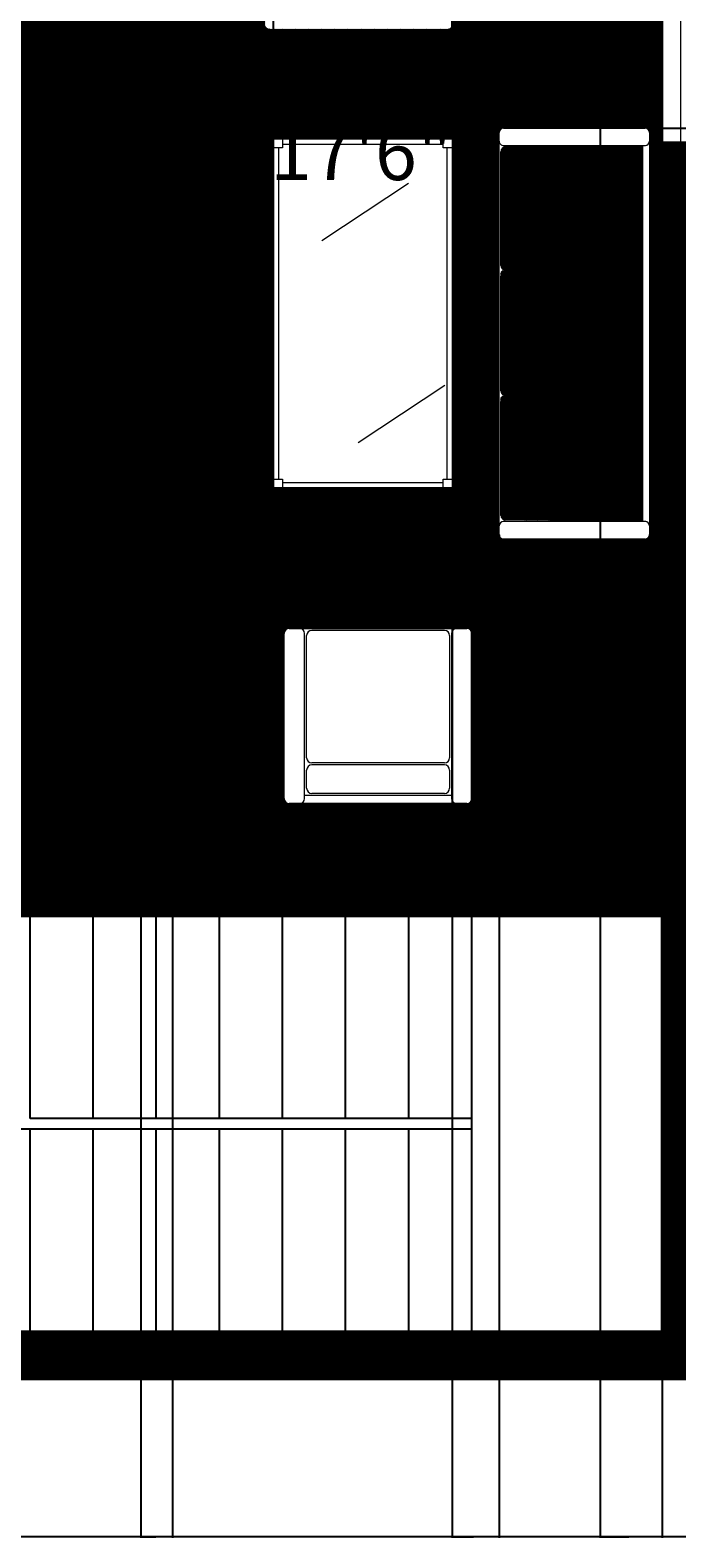
# Model space of a CAD drawing. Units: inches. Extents: x 205 to 1667, y -23 to 828.
# Tile 4 of 10: x 645 to 768, y -23 to 264. Entities that reach past the tile are written whole.
import ezdxf

# ---------------------------------------------------------------- set-up
doc = ezdxf.new("R2010")
doc.units = ezdxf.units.IN
doc.header["$MEASUREMENT"] = 0
for name, color, linetype, lineweight in [('A-ANNO-DIMS', 2, 'Continuous', 18), ('A-AREA-IDEN', 7, 'Continuous', 25), ('A-FLOR-STRS', 7, 'Continuous', 25), ('A-FURN', 8, 'Continuous', 18), ('A-GLAZ', 4, 'Continuous', 18), ('A-WALL', 7, 'Continuous', 35)]:
    doc.layers.add(name, color=color, linetype=linetype, lineweight=lineweight)
doc.layers.add('A-FLOR-PATT', color=9, linetype='Continuous', lineweight=9, true_color=0xc7c8ca)
doc.styles.get("Standard").update_dxf_attribs({"font": 'arial.ttf'})
doc.dimstyles.get("Standard").update_dxf_attribs({"dimtxt": 0.18, "dimasz": 0.18, "dimexe": 0.18, "dimexo": 0.0625, "dimgap": 0.09, "dimtad": 0, "dimtih": 1, "dimtoh": 1, "dimdec": 4, "dimzin": 0, "dimdsep": 46, "dimtxsty": 'Standard', "dimcen": 0.09, "dimadec": 0, "dimazin": 0, "dimtfac": 1, "dimtdec": 4, "dimtofl": 0, "dimtmove": 0, "dimatfit": 3, "dimfxl": 1, "dimtolj": 1, "dimtzin": 0, "dimarcsym": 0})

# ---------------------------------------------------------------- blocks, each defined once
blk = doc.blocks.new('A$C0BA509B0')
for p, q in [((0, 0.025), (0, 0.835)), ((0.025, 0.86), (2.325, 0.86)), ((0.1, 0.0219), (0.1, 0.8375)), ((0.1, 0.82), (2.25, 0.82)), ((0.11, 0.695), (0.11, 0.785)), ((0.135, 0.81), (0.7866, 0.81)), ((0.8116, 0.785), (0.8116, 0.695)), ((0.8216, 0.785), (0.8216, 0.695)), ((0.8466, 0.81), (1.5033, 0.81)), ((1.5283, 0.785), (1.5283, 0.695)), ((1.5383, 0.785), (1.5383, 0.695)), ((1.5633, 0.81), (2.215, 0.81)), ((2.24, 0.785), (2.24, 0.695)), ((2.25, 0.8385), (2.25, 0.0224)), ((2.35, 0.835), (2.35, 0.025)), ((0.11, 0.035), (0.11, 0.635)), ((0.135, 0.67), (0.7866, 0.67)), ((0.135, 0.66), (0.7866, 0.66)), ((0.8116, 0.635), (0.8116, 0.035)), ((0.8216, 0.635), (0.8216, 0.035)), ((0.8466, 0.67), (1.5033, 0.67)), ((0.8466, 0.66), (1.5033, 0.66)), ((1.5283, 0.635), (1.5283, 0.035)), ((1.5383, 0.635), (1.5383, 0.035)), ((1.5633, 0.67), (2.215, 0.67)), ((1.5633, 0.66), (2.215, 0.66)), ((2.24, 0.635), (2.24, 0.035)), ((0.7866, 0.01), (0.135, 0.01)), ((1.5033, 0.01), (0.8466, 0.01)), ((2.215, 0.01), (1.5633, 0.01)), ((2.325, 0), (0.025, 0))]:
    blk.add_line(p, q)
for centre, start, end in [((0.025, 0.835), 90, 180), ((0.0751, 0.835), 0, 90), ((0.135, 0.785), 90, 180), ((0.7866, 0.785), 0, 90), ((0.8466, 0.785), 90, 180), ((1.5033, 0.785), 0, 90), ((1.5633, 0.785), 90, 180), ((2.215, 0.785), 0, 90), ((2.2752, 0.835), 90, 180), ((2.325, 0.835), 0, 90), ((0.135, 0.695), 180, 270), ((0.7866, 0.695), 270, 0), ((0.8466, 0.695), 180, 270), ((1.5033, 0.695), 270, 0), ((1.5633, 0.695), 180, 270), ((2.215, 0.695), 270, 0), ((0.135, 0.635), 90, 180), ((0.7866, 0.635), 0, 90), ((0.8466, 0.635), 90, 180), ((1.5033, 0.635), 0, 90), ((1.5633, 0.635), 90, 180), ((2.215, 0.635), 0, 90), ((0.025, 0.025), 180, 270), ((0.0751, 0.025), 270, 0), ((0.135, 0.035), 180, 270), ((0.7866, 0.035), 270, 0), ((0.8466, 0.035), 180, 270), ((1.5033, 0.035), 270, 0), ((1.5633, 0.035), 180, 270), ((2.215, 0.035), 270, 0), ((2.2749, 0.025), 180, 270), ((2.325, 0.025), 270, 0)]:
    blk.add_arc(centre, 0.025, start, end)
blk = doc.blocks.new('WIN-48IN')
for p, q in [((0, 0), (0, 9)), ((0, 9), (48, 9)), ((48, 9), (48, 0)), ((48, 5.5), (0, 5.5)), ((48, 3.5), (0, 3.5)), ((48, 0), (0, 0))]:
    blk.add_line(p, q)
blk = doc.blocks.new('CHAIR-LOUNGE')
for p, q in [((0, 0.97), (0, 32.36)), ((0.97, 33.33), (34.75, 33.33)), ((3.88, 0.83), (3.88, 32.46)), ((4.26, 8.72), (4.26, 31.94)), ((30.48, 32.94), (5.26, 32.94)), ((31.45, 31.97), (31.45, 8.72)), ((31.84, 32.48), (31.84, 0.87)), ((35.71, 32.36), (35.71, 0.97)), ((4.26, 2.91), (4.26, 6.39)), ((30.48, 7.75), (5.23, 7.75)), ((30.48, 7.36), (5.23, 7.36)), ((31.45, 6.39), (31.45, 2.91)), ((31.84, 1.55), (3.88, 1.55)), ((30.48, 1.94), (5.23, 1.94)), ((34.75, 0), (0.97, 0))]:
    blk.add_line(p, q)
for centre, radius, start, end in [((0.97, 32.36), 0.969, 90, 180), ((2.91, 32.36), 0.969, 0, 90), ((5.26, 31.94), 1, 90, 180), ((5.23, 31.97), 0.969, 169.6161, 180), ((30.48, 31.97), 0.969, 0, 90), ((32.8, 32.36), 0.969, 90, 180), ((34.75, 32.36), 0.969, 0, 90), ((5.23, 8.72), 0.969, 180, 270), ((30.48, 8.72), 0.969, 270, 0), ((5.23, 6.39), 0.969, 90, 180), ((30.48, 6.39), 0.969, 0, 90), ((5.23, 2.91), 0.969, 180, 270), ((30.48, 2.91), 0.969, 270, 0), ((0.97, 0.97), 0.969, 180, 270), ((2.9, 0.97), 0.969, 270, 0), ((32.8, 0.97), 0.969, 180, 270), ((34.75, 0.97), 0.969, 270, 0)]:
    blk.add_arc(centre, radius, start, end)
blk = doc.blocks.new('*D22')
at = {"layer": 'A-ANNO-DIMS', "color": 0, "lineweight": -2, "transparency": 16777216}
for p, q in [((693.55, 116.97), (693.55, 111.5)), ((729.26, 116.97), (729.26, 111.5)), ((693.73, 111.68), (710.45, 111.68)), ((729.08, 111.68), (712.36, 111.68))]:
    blk.add_line(p, q, dxfattribs=at)
at = {"layer": 'A-ANNO-DIMS', "color": 0, "transparency": 16777216}
for points in [[(693.73, 111.71), (693.73, 111.65), (693.55, 111.68)], [(729.08, 111.71), (729.08, 111.65), (729.26, 111.68)]]:
    blk.add_solid(points, dxfattribs=at)
at = {"layer": 'Defpoints', "color": 0, "transparency": 16777216}
for p in [(693.55, 117.03), (729.26, 117.03), (729.26, 111.68)]:
    blk.add_point(p, dxfattribs=at)
at = {"layer": 'A-ANNO-DIMS', "color": 0, "transparency": 16777216, "insert": (711.4, 111.68), "char_height": 0.18, "attachment_point": 5}
blk.add_mtext('\\A1;CHAIR 36 TYP.', dxfattribs=at)
blk = doc.blocks.new('*D23')
at = {"layer": 'A-ANNO-DIMS', "color": 0, "lineweight": -2, "transparency": 16777216}
for p, q in [((729.32, 150.36), (734.8, 150.36)), ((734.62, 150.18), (734.62, 133.88)), ((734.62, 117.21), (734.62, 133.52)), ((729.32, 117.03), (734.8, 117.03))]:
    blk.add_line(p, q, dxfattribs=at)
at = {"layer": 'A-ANNO-DIMS', "color": 0, "transparency": 16777216}
for points in [[(734.59, 150.18), (734.65, 150.18), (734.62, 150.36)], [(734.59, 117.21), (734.65, 117.21), (734.62, 117.03)]]:
    blk.add_solid(points, dxfattribs=at)
at = {"layer": 'Defpoints', "color": 0, "transparency": 16777216}
for p in [(729.26, 150.36), (734.62, 150.36), (729.26, 117.03)]:
    blk.add_point(p, dxfattribs=at)
at = {"layer": 'A-ANNO-DIMS', "color": 0, "transparency": 16777216, "insert": (734.62, 133.7), "char_height": 0.18, "attachment_point": 5}
blk.add_mtext('\\A1;33 TYP.', dxfattribs=at)
blk = doc.blocks.new('*D34')
at = {"layer": 'A-ANNO-DIMS', "color": 0, "lineweight": -2, "transparency": 16777216}
for p, q in [((638.54, 153.38), (645.08, 153.38)), ((644.9, 153.2), (644.9, 132.17)), ((644.9, 110.77), (644.9, 131.8)), ((638.54, 110.59), (645.08, 110.59))]:
    blk.add_line(p, q, dxfattribs=at)
at = {"layer": 'A-ANNO-DIMS', "color": 0, "transparency": 16777216}
for points in [[(644.87, 153.2), (644.93, 153.2), (644.9, 153.38)], [(644.87, 110.77), (644.93, 110.77), (644.9, 110.59)]]:
    blk.add_solid(points, dxfattribs=at)
at = {"layer": 'Defpoints', "color": 0, "transparency": 16777216}
for p in [(638.48, 153.38), (644.9, 153.38), (638.48, 110.59)]:
    blk.add_point(p, dxfattribs=at)
at = {"layer": 'A-ANNO-DIMS', "color": 0, "transparency": 16777216, "insert": (644.9, 131.98), "char_height": 0.18, "attachment_point": 5}
blk.add_mtext('\\A1;PAIRED DOOR 43', dxfattribs=at)
blk = doc.blocks.new('*D38')
at = {"layer": 'A-ANNO-DIMS', "color": 0, "lineweight": -2, "transparency": 16777216}
for p, q in [((763.1, 245.49), (774.93, 245.49)), ((774.75, 245.31), (774.75, 206.61)), ((774.75, 167.53), (774.75, 206.24)), ((763.1, 167.35), (774.93, 167.35))]:
    blk.add_line(p, q, dxfattribs=at)
at = {"layer": 'A-ANNO-DIMS', "color": 0, "transparency": 16777216}
for points in [[(774.72, 245.31), (774.78, 245.31), (774.75, 245.49)], [(774.72, 167.53), (774.78, 167.53), (774.75, 167.35)]]:
    blk.add_solid(points, dxfattribs=at)
at = {"layer": 'Defpoints', "color": 0, "transparency": 16777216}
for p in [(763.03, 245.49), (763.03, 167.35), (774.75, 167.35)]:
    blk.add_point(p, dxfattribs=at)
at = {"layer": 'A-ANNO-DIMS', "color": 0, "transparency": 16777216, "insert": (774.75, 206.42), "char_height": 0.18, "attachment_point": 5}
blk.add_mtext('\\A1;SOFA 78', dxfattribs=at)
blk = doc.blocks.new('*D39')
at = {"layer": 'A-ANNO-DIMS', "color": 0, "lineweight": -2, "transparency": 16777216}
for p, q in [((734.44, 245.56), (734.44, 257.39)), ((734.62, 257.21), (748.51, 257.21)), ((762.85, 257.21), (748.96, 257.21)), ((763.03, 245.56), (763.03, 257.39))]:
    blk.add_line(p, q, dxfattribs=at)
at = {"layer": 'A-ANNO-DIMS', "color": 0, "transparency": 16777216}
for points in [[(734.62, 257.24), (734.62, 257.18), (734.44, 257.21)], [(762.85, 257.24), (762.85, 257.18), (763.03, 257.21)]]:
    blk.add_solid(points, dxfattribs=at)
at = {"layer": 'Defpoints', "color": 0, "transparency": 16777216}
for p in [(763.03, 257.21), (734.44, 245.49), (763.03, 245.49)]:
    blk.add_point(p, dxfattribs=at)
at = {"layer": 'A-ANNO-DIMS', "color": 0, "transparency": 16777216, "insert": (748.74, 257.21), "char_height": 0.18, "attachment_point": 5}
blk.add_mtext('\\A1;29', dxfattribs=at)
blk = doc.blocks.new('*D42')
at = {"layer": 'A-ANNO-DIMS', "color": 0, "lineweight": -2, "transparency": 16777216}
for p, q in [((462.43, 7.59), (462.43, -22.59)), ((774.43, 7.59), (774.43, -22.59)), ((462.61, -22.41), (618.14, -22.41)), ((774.25, -22.41), (618.72, -22.41))]:
    blk.add_line(p, q, dxfattribs=at)
at = {"layer": 'A-ANNO-DIMS', "color": 0, "transparency": 16777216}
for points in [[(462.61, -22.38), (462.61, -22.44), (462.43, -22.41)], [(774.25, -22.38), (774.25, -22.44), (774.43, -22.41)]]:
    blk.add_solid(points, dxfattribs=at)
at = {"layer": 'Defpoints', "color": 0, "transparency": 16777216}
for p in [(462.43, 7.65), (774.43, 7.65), (774.43, -22.41)]:
    blk.add_point(p, dxfattribs=at)
at = {"layer": 'A-ANNO-DIMS', "color": 0, "transparency": 16777216, "insert": (618.43, -22.41), "char_height": 0.18, "attachment_point": 5}
blk.add_mtext('\\A1;312', dxfattribs=at)
blk = doc.blocks.new('*D45')
at = {"layer": 'A-ANNO-DIMS', "color": 0, "lineweight": -2, "transparency": 16777216}
for p, q in [((765.49, 95.64), (804.67, 95.64)), ((804.49, 95.46), (804.49, 51.83)), ((804.49, 7.83), (804.49, 51.46)), ((774.49, 7.65), (804.67, 7.65))]:
    blk.add_line(p, q, dxfattribs=at)
at = {"layer": 'A-ANNO-DIMS', "color": 0, "transparency": 16777216}
for points in [[(804.46, 95.46), (804.52, 95.46), (804.49, 95.64)], [(804.46, 7.83), (804.52, 7.83), (804.49, 7.65)]]:
    blk.add_solid(points, dxfattribs=at)
at = {"layer": 'Defpoints', "color": 0, "transparency": 16777216}
for p in [(765.43, 95.64), (804.49, 95.64), (774.43, 7.65)]:
    blk.add_point(p, dxfattribs=at)
at = {"layer": 'A-ANNO-DIMS', "color": 0, "transparency": 16777216, "insert": (804.49, 51.64), "char_height": 0.18, "attachment_point": 5}
blk.add_mtext('\\A1;87.99', dxfattribs=at)
blk = doc.blocks.new('*D54')
at = {"layer": 'A-ANNO-DIMS', "color": 0, "lineweight": -2, "transparency": 16777216}
for p, q in [((729.22, 16.71), (729.22, 637.89)), ((729.4, 637.71), (746.95, 637.71)), ((765.25, 637.71), (747.7, 637.71)), ((765.43, 16.71), (765.43, 637.89))]:
    blk.add_line(p, q, dxfattribs=at)
at = {"layer": 'A-ANNO-DIMS', "color": 0, "transparency": 16777216}
for points in [[(729.4, 637.74), (729.4, 637.68), (729.22, 637.71)], [(765.25, 637.74), (765.25, 637.68), (765.43, 637.71)]]:
    blk.add_solid(points, dxfattribs=at)
at = {"layer": 'Defpoints', "color": 0, "transparency": 16777216}
for p in [(729.22, 637.71), (729.22, 16.65), (765.43, 16.65)]:
    blk.add_point(p, dxfattribs=at)
at = {"layer": 'A-ANNO-DIMS', "color": 0, "transparency": 16777216, "insert": (747.33, 637.71), "char_height": 0.18, "attachment_point": 5}
blk.add_mtext('\\A1;36.21', dxfattribs=at)
blk = doc.blocks.new('*D61')
at = {"layer": 'A-ANNO-DIMS', "color": 0, "lineweight": -2, "transparency": 16777216}
for p, q in [((666.3, 319.88), (666.3, -22.59)), ((672.3, 319.88), (672.3, -22.59)), ((666.48, -22.41), (669.15, -22.41)), ((672.12, -22.41), (669.45, -22.41))]:
    blk.add_line(p, q, dxfattribs=at)
at = {"layer": 'A-ANNO-DIMS', "color": 0, "transparency": 16777216}
for points in [[(666.48, -22.38), (666.48, -22.44), (666.3, -22.41)], [(672.12, -22.38), (672.12, -22.44), (672.3, -22.41)]]:
    blk.add_solid(points, dxfattribs=at)
at = {"layer": 'Defpoints', "color": 0, "transparency": 16777216}
for p in [(666.3, 319.94), (672.3, 319.94), (672.3, -22.41)]:
    blk.add_point(p, dxfattribs=at)
at = {"layer": 'A-ANNO-DIMS', "color": 0, "transparency": 16777216, "insert": (669.3, -22.41), "char_height": 0.18, "attachment_point": 5}
blk.add_mtext('\\A1;6', dxfattribs=at)
blk = doc.blocks.new('*D63')
at = {"layer": 'A-ANNO-DIMS', "color": 0, "lineweight": -2, "transparency": 16777216}
for p, q in [((753.65, 320.09), (753.65, -22.59)), ((765.43, 319.88), (765.43, -22.59)), ((753.83, -22.41), (759.09, -22.41)), ((765.25, -22.41), (760, -22.41))]:
    blk.add_line(p, q, dxfattribs=at)
at = {"layer": 'A-ANNO-DIMS', "color": 0, "transparency": 16777216}
for points in [[(753.83, -22.38), (753.83, -22.44), (753.65, -22.41)], [(765.25, -22.38), (765.25, -22.44), (765.43, -22.41)]]:
    blk.add_solid(points, dxfattribs=at)
at = {"layer": 'Defpoints', "color": 0, "transparency": 16777216}
for p in [(753.65, 320.15), (765.43, 319.94), (753.65, -22.41)]:
    blk.add_point(p, dxfattribs=at)
at = {"layer": 'A-ANNO-DIMS', "color": 0, "transparency": 16777216, "insert": (759.54, -22.41), "char_height": 0.18, "attachment_point": 5}
blk.add_mtext('\\A1;11.778', dxfattribs=at)
blk = doc.blocks.new('*D66')
at = {"layer": 'A-ANNO-DIMS', "color": 0, "lineweight": -2, "transparency": 16777216}
for p, q in [((691.51, 243.5), (691.51, 637.89)), ((691.69, 637.71), (708.11, 637.71)), ((725.32, 637.71), (708.9, 637.71)), ((725.5, 243.5), (725.5, 637.89))]:
    blk.add_line(p, q, dxfattribs=at)
at = {"layer": 'A-ANNO-DIMS', "color": 0, "transparency": 16777216}
for points in [[(691.69, 637.74), (691.69, 637.68), (691.51, 637.71)], [(725.32, 637.74), (725.32, 637.68), (725.5, 637.71)]]:
    blk.add_solid(points, dxfattribs=at)
at = {"layer": 'Defpoints', "color": 0, "transparency": 16777216}
for p in [(725.5, 637.71), (691.51, 243.44), (725.5, 243.44)]:
    blk.add_point(p, dxfattribs=at)
at = {"layer": 'A-ANNO-DIMS', "color": 0, "transparency": 16777216, "insert": (708.5, 637.71), "char_height": 0.18, "attachment_point": 5}
blk.add_mtext('\\A1;33.99', dxfattribs=at)
blk = doc.blocks.new('*D67')
at = {"layer": 'A-ANNO-DIMS', "color": 0, "lineweight": -2, "transparency": 16777216}
for p, q in [((691.44, 243.44), (432.19, 243.44)), ((432.37, 243.26), (432.37, 210.43)), ((432.37, 177.23), (432.37, 210.06)), ((691.44, 177.05), (432.19, 177.05))]:
    blk.add_line(p, q, dxfattribs=at)
at = {"layer": 'A-ANNO-DIMS', "color": 0, "transparency": 16777216}
for points in [[(432.34, 243.26), (432.4, 243.26), (432.37, 243.44)], [(432.34, 177.23), (432.4, 177.23), (432.37, 177.05)]]:
    blk.add_solid(points, dxfattribs=at)
at = {"layer": 'Defpoints', "color": 0, "transparency": 16777216}
for p in [(432.37, 243.44), (691.51, 243.44), (691.51, 177.05)]:
    blk.add_point(p, dxfattribs=at)
at = {"layer": 'A-ANNO-DIMS', "color": 0, "transparency": 16777216, "insert": (432.37, 210.24), "char_height": 0.18, "attachment_point": 5}
blk.add_mtext('\\A1;66.39', dxfattribs=at)
blk = doc.blocks.new('*D68')
at = {"layer": 'A-ANNO-DIMS', "color": 0, "lineweight": -2, "transparency": 16777216}
for p, q in [((626.35, 153.44), (626.35, 637.89)), ((626.53, 637.71), (658.53, 637.71)), ((691.33, 637.71), (659.32, 637.71)), ((691.51, 177.11), (691.51, 637.89))]:
    blk.add_line(p, q, dxfattribs=at)
at = {"layer": 'A-ANNO-DIMS', "color": 0, "transparency": 16777216}
for points in [[(626.53, 637.74), (626.53, 637.68), (626.35, 637.71)], [(691.33, 637.74), (691.33, 637.68), (691.51, 637.71)]]:
    blk.add_solid(points, dxfattribs=at)
at = {"layer": 'Defpoints', "color": 0, "transparency": 16777216}
for p in [(626.35, 637.71), (691.51, 177.05), (626.35, 153.38)]:
    blk.add_point(p, dxfattribs=at)
at = {"layer": 'A-ANNO-DIMS', "color": 0, "transparency": 16777216, "insert": (658.93, 637.71), "char_height": 0.18, "attachment_point": 5}
blk.add_mtext('\\A1;65.16', dxfattribs=at)
blk = doc.blocks.new('*D69')
at = {"layer": 'A-ANNO-DIMS', "color": 0, "lineweight": -2, "transparency": 16777216}
for p, q in [((725.5, 176.99), (725.5, -22.59)), ((734.44, 168.12), (734.44, -22.59)), ((725.68, -22.41), (729.57, -22.41)), ((734.26, -22.41), (730.36, -22.41))]:
    blk.add_line(p, q, dxfattribs=at)
at = {"layer": 'A-ANNO-DIMS', "color": 0, "transparency": 16777216}
for points in [[(725.68, -22.38), (725.68, -22.44), (725.5, -22.41)], [(734.26, -22.38), (734.26, -22.44), (734.44, -22.41)]]:
    blk.add_solid(points, dxfattribs=at)
at = {"layer": 'Defpoints', "color": 0, "transparency": 16777216}
for p in [(725.5, 177.05), (734.44, 168.18), (734.44, -22.41)]:
    blk.add_point(p, dxfattribs=at)
at = {"layer": 'A-ANNO-DIMS', "color": 0, "transparency": 16777216, "insert": (729.97, -22.41), "char_height": 0.18, "attachment_point": 5}
blk.add_mtext('\\A1;8.939', dxfattribs=at)
blk = doc.blocks.new('*D70')
at = {"layer": 'A-ANNO-DIMS', "color": 0, "lineweight": -2, "transparency": 16777216}
for p, q in [((729.04, 117.32), (804.67, 117.32)), ((804.49, 117.14), (804.49, 111.16)), ((804.49, 104.82), (804.49, 110.8)), ((765.49, 104.64), (804.67, 104.64))]:
    blk.add_line(p, q, dxfattribs=at)
at = {"layer": 'A-ANNO-DIMS', "color": 0, "transparency": 16777216}
for points in [[(804.46, 117.14), (804.52, 117.14), (804.49, 117.32)], [(804.46, 104.82), (804.52, 104.82), (804.49, 104.64)]]:
    blk.add_solid(points, dxfattribs=at)
at = {"layer": 'Defpoints', "color": 0, "transparency": 16777216}
for p in [(728.98, 117.32), (804.49, 117.32), (765.43, 104.64)]:
    blk.add_point(p, dxfattribs=at)
at = {"layer": 'A-ANNO-DIMS', "color": 0, "transparency": 16777216, "insert": (804.49, 110.98), "char_height": 0.18, "attachment_point": 5}
blk.add_mtext('\\A1;12.68', dxfattribs=at)

msp = doc.modelspace()

# ---------------------------------------------------------------- hatches: boundary and pattern name
at = {"layer": 'A-FLOR-PATT'}
h = msp.add_hatch(dxfattribs=at)
h.set_pattern_fill('ANSI31', color=256)
h.paths.add_polyline_path([(774.4305, 607.6511), (720.5338, 607.6511), (720.5338, 598.6511), (727.9933, 598.6511), (746.8614, 598.6511), (765.4305, 598.6511), (765.4305, 454.6511), (759.5298, 454.6511), (759.5298, 448.9635), (765.4305, 448.9635), (765.4305, 428.0602), (774.4305, 428.0602)])
h.paths.add_polyline_path([(765.4305, 598.6511), (746.8614, 598.6511), (746.8614, 579.7829), (727.9933, 579.7829), (727.9933, 518.1387, -0.41421701), (724.6389, 514.7843), (668.2693, 514.7843, -0.41421356), (665.0743, 517.9793), (665.0743, 579.7829), (646.2062, 579.7829), (646.2062, 598.6511), (626.3468, 598.6511), (626.3468, 454.6511), (628.3468, 454.6511), (628.3468, 484.9635, -0.41421356), (664.3468, 449.9635), (664.3468, 454.6511), (729.3305, 454.6511), (758.5298, 454.6511), (759.5298, 454.6511), (765.4305, 454.6511)])
h.paths.add_polyline_path([(621.4404, 598.6511), (471.4305, 598.6511), (471.4305, 568.8442), (490.2987, 568.8442), (490.2987, 549.9761), (551.9429, 549.9761, -0.41421701), (555.2973, 546.6217), (555.2973, 490.2521, -0.41421356), (552.1023, 487.0571), (490.2987, 487.0571), (490.2987, 468.189), (471.4305, 468.189), (471.4305, 454.6511), (583.4404, 454.6511), (583.4404, 449.9635, -0.41421356), (619.4404, 484.9635), (619.4404, 454.6511), (621.4404, 454.6511)])
h.paths.add_polyline_path([(672.5338, 607.6511), (569.5707, 607.6511), (569.5707, 598.6511), (621.4404, 598.6511), (621.4404, 454.6511), (619.4404, 454.6511), (619.4404, 448.9635), (628.3468, 448.9635), (628.3468, 454.6511), (626.3468, 454.6511), (626.3468, 598.6511), (646.2062, 598.6511), (665.0743, 598.6511), (672.5338, 598.6511)])
h.paths.add_polyline_path([(521.5707, 607.6511), (462.4305, 607.6511), (462.4305, 407.4306), (471.4305, 407.4306), (471.4305, 448.9635), (583.4404, 448.9635, -0.0070419), (583.4404, 449.9635), (583.4404, 454.6511), (471.4305, 454.6511), (471.4305, 468.189), (471.4305, 487.0571), (471.4305, 549.9761), (471.4305, 568.8442), (471.4305, 598.6511), (521.5707, 598.6511)])
h.paths.add_polyline_path([(471.4305, 314.3187), (583.4404, 314.3187), (583.4404, 319.9388), (471.4305, 319.9388), (471.4305, 359.4306), (462.4305, 359.4306), (462.4305, 7.6511), (471.4305, 7.6511), (471.4305, 204.9321), (521.9355, 204.9321), (521.9355, 213.9321), (471.4305, 213.9321)])
h.paths.add_polyline_path([(774.4305, 410.0602), (765.4305, 410.0602), (765.4305, 389.1569), (672.3024, 389.1569), (672.3024, 448.9635), (681.1739, 448.9635, -0.18532444), (681.6564, 449.1487), (698.6035, 449.1487), (729.3305, 448.9635), (729.3305, 454.6511), (664.3468, 454.6511), (664.3468, 449.9635, -0.0070419), (664.3468, 448.9635), (666.3024, 448.9635), (666.3024, 378.2485), (672.3024, 378.2485), (672.3024, 383.1306), (765.4305, 383.1306), (765.4305, 360.5347), (774.4305, 360.5347)])
h.paths.add_polyline_path([(774.4305, 342.5347), (765.4305, 342.5347), (765.4305, 319.9388), (672.3024, 319.9388), (672.3024, 348.5574), (671.0896, 348.5574, -0.04071533), (666.3024, 348.2485), (666.3024, 319.9388), (664.3468, 319.9388, -0.0070419), (664.3468, 318.9388), (664.3468, 314.3187), (765.4305, 314.3187), (765.4305, 290.8426), (774.4305, 290.8426)])
h.paths.add_polyline_path([(774.4305, 242.8426), (765.4305, 242.8426), (765.4305, 104.6382), (626.3468, 104.6382), (626.3468, 110.5917), (617.3468, 110.5917), (617.3468, 95.6382), (765.4305, 95.6382), (765.4305, 16.6511), (621.2232, 16.6511), (621.2232, 7.6511), (774.4305, 7.6511)])
h.paths.add_polyline_path([(626.3468, 314.3187), (628.3468, 314.3187), (628.3468, 319.9388), (619.4404, 319.9388), (619.4404, 314.3187), (620.4404, 314.3187), (620.4404, 213.9321), (569.9355, 213.9321), (569.9355, 204.9321), (617.3468, 204.9321), (617.3468, 153.3751), (626.3468, 153.3751)])
h.paths.add_polyline_path([(620.4404, 314.3187), (619.4404, 314.3187), (619.4404, 319.9388), (628.3468, 319.9388), (629.3468, 319.9388), (629.3468, 283.9388, 0.40598745), (664.3468, 318.9388), (664.3468, 319.9388), (666.3024, 319.9388), (666.3024, 348.2485), (666.3024, 377.2485), (666.3024, 378.2485), (666.3024, 448.9635), (664.3468, 448.9635), (664.3468, 449.9635, 0.40598745), (629.3468, 484.9635), (629.3468, 448.9635), (628.3468, 448.9635), (619.4404, 448.9635), (618.4404, 448.9635), (618.4404, 484.9635, 0.40598745), (583.4404, 449.9635), (583.4404, 448.9635), (471.4305, 448.9635), (471.4305, 407.4306), (471.4305, 359.4306), (471.4305, 319.9388), (583.4404, 319.9388), (583.4404, 314.3187), (495.4305, 314.3187), (495.4305, 237.9321), (620.4404, 237.9321)])
h.paths.add_polyline_path([(525.0876, 347.7863), (513.5657, 347.7863), (512.0216, 362.1672), (526.6317, 362.1672)], flags=16)
h.paths.add_polyline_path([(550.9499, 370.1471), (536.569, 368.6029), (536.569, 383.2131), (550.9499, 381.6689)], flags=16)
h.paths.add_polyline_path([(530.7713, 364.5431), (508.0415, 364.5431, -0.41421356), (504.7944, 367.7902), (504.7944, 403.5085, -0.41421356), (508.0415, 406.7556), (530.7713, 406.7556, -0.41421356), (534.0184, 403.5085), (534.0184, 367.7902, -0.41421356)], flags=16)
h.paths.add_polyline_path([(550.9499, 389.6298), (536.569, 388.0856), (536.569, 402.6958), (550.9499, 401.1516)], flags=16)
h.paths.add_polyline_path([(502.2439, 368.6029), (487.863, 370.1471), (487.863, 381.6689), (502.2439, 383.2131)], flags=16)
h.paths.add_polyline_path([(502.2439, 388.0856), (487.863, 389.6298), (487.863, 401.1516), (502.2439, 402.6958)], flags=16)
h.paths.add_polyline_path([(526.6317, 409.1315), (512.0216, 409.1315), (513.5657, 423.5124), (525.0876, 423.5124)], flags=16)
h.paths.add_polyline_path([(765.4305, 290.8426), (765.4305, 314.3187), (664.3468, 314.3187), (664.3468, 318.9388, -0.41421356), (628.3468, 283.9388), (628.3468, 314.3187), (626.3468, 314.3187), (626.3468, 153.3751), (638.3468, 153.3751, -0.4196361), (617.5748, 131.9834, -0.4196361), (638.3468, 110.5917), (626.3468, 110.5917), (626.3468, 104.6382), (765.4305, 104.6382), (765.4305, 242.8426)])
h.paths.add_polyline_path([(691.5064, 243.4363), (693.2483, 243.4363), (725.4984, 243.4363), (725.4984, 241.7329), (725.4984, 177.0512), (723.7564, 177.0512), (691.5064, 177.0512), (691.5064, 178.7545)], flags=16)
h.paths.add_polyline_path([(689.8658, 265.2977), (689.8658, 296.6873, -0.41421356), (690.8346, 297.6561), (724.6111, 297.6561, -0.41421356), (725.5799, 296.6873), (725.5799, 265.2977, -0.41421356), (724.6111, 264.3289), (690.8346, 264.3289, -0.41421356)], flags=16)
h.paths.add_polyline_path([(694.1286, 265.6852), (694.1286, 288.9368, -0.41421356), (695.0974, 289.9056), (720.3483, 289.9056, -0.41421356), (721.3171, 288.9368), (721.3171, 265.6852, -0.04533947), (721.3013, 265.5106, -0.3531705), (720.3282, 264.7164), (695.0974, 264.7164, -0.41421356)], flags=0)
h.paths.add_polyline_path([(694.1286, 291.2619), (694.1286, 294.7497, -0.41421356), (695.0974, 295.7185), (720.3483, 295.7185, -0.41421356), (721.3171, 294.7497), (721.3171, 291.2619, -0.41421356), (720.3483, 290.2931), (695.0974, 290.2931, -0.41421356)], flags=0)
h.paths.add_polyline_path([(734.4369, 244.6615, -0.41421356), (735.2682, 245.4928), (762.2019, 245.4928, -0.41421356), (763.0332, 244.6615), (763.0332, 168.183, -0.41421356), (762.2019, 167.3517), (735.2682, 167.3517, -0.41421356), (734.4369, 168.183)], flags=16)
h.paths.add_polyline_path([(761.7032, 242.1676), (761.7032, 170.6768), (735.6007, 171.0093, -0.41421356), (734.7694, 171.8406), (734.7694, 193.5102, -0.56972741), (735.6007, 194.674, -0.41421356), (734.7694, 195.5053), (734.7694, 217.3423, -0.56972741), (735.6007, 218.5061, -0.41421356), (734.7694, 219.3374), (734.7694, 241.0038, -0.41421356), (735.6007, 241.8351), (735.1643, 242.1676)], flags=16)
h.paths.add_polyline_path([(757.5467, 171.0093), (760.5393, 171.0093, 0.41421356), (761.3706, 171.8406), (761.3706, 193.5102, 0.41421356), (760.5393, 194.3415), (757.5467, 194.3415, 0.41421356), (756.7154, 193.5102), (756.7155, 171.8534, 0.41871477)], flags=0)
h.paths.add_polyline_path([(756.7154, 241.0038, -0.41421356), (757.5467, 241.8351), (760.5393, 241.8351, -0.41421356), (761.3706, 241.0038), (761.3706, 219.3374, -0.41421356), (760.5393, 218.5061), (760.5393, 218.1736, -0.41421356), (761.3706, 217.3423), (761.3706, 195.5053, -0.41421356), (760.5393, 194.674), (757.5467, 194.674, -0.56972741), (756.3829, 195.5053, -0.41421356), (755.5516, 194.674), (755.5516, 194.3415, -0.41421356), (756.3829, 193.5102), (756.7154, 171.8406), (756.3829, 193.5102, 0.41421356), (755.5516, 194.3415), (735.6007, 194.674), (755.5516, 194.674, 0.41421356), (756.3829, 195.5053), (756.3829, 217.3423, 0.41421356), (755.5516, 218.1736), (735.6007, 218.5061), (755.5516, 218.5061, 0.41421356), (756.3829, 219.3374)], flags=0)
h.paths.add_polyline_path([(694.5151, 150.3608), (728.2916, 150.3608, -0.41421356), (729.2604, 149.3919), (729.2604, 118.0023, -0.41421356), (728.2916, 117.0335), (694.5151, 117.0335, -0.41421356), (693.5463, 118.0023), (693.5463, 149.3919, -0.41421356)], flags=16)
h.paths.add_polyline_path([(724.0288, 149.9732, -0.41421356), (724.9977, 149.0044), (724.9977, 125.7529, -0.41421356), (724.0288, 124.784), (698.7779, 124.784, -0.41421356), (697.8091, 125.7529), (697.8091, 149.0044, -0.04533947), (697.825, 149.179, -0.3531705), (698.798, 149.9732)], flags=0)
h.paths.add_polyline_path([(698.7779, 124.3965), (724.0288, 124.3965, -0.41421356), (724.9977, 123.4277), (724.9977, 119.94, -0.41421356), (724.0288, 118.9711), (698.7779, 118.9711, -0.41421356), (697.8091, 119.94), (697.8091, 123.4277, -0.41421356)], flags=0)

# ---------------------------------------------------------------- linework, layer by layer
at = {"layer": 'A-FLOR-STRS'}
for p, q in [((645.2232, 57.1446), (645.2232, 95.6382)), ((657.2232, 57.1446), (657.2232, 95.6382)), ((669.2232, 57.1446), (669.2232, 95.6382)), ((681.2232, 57.1446), (681.2232, 95.6382)), ((693.2232, 57.1446), (693.2232, 95.6382)), ((705.2232, 57.1446), (705.2232, 95.6382)), ((717.2232, 57.1446), (717.2232, 95.6382)), ((729.2232, 16.6511), (729.2232, 95.6382)), ((729.2232, 55.1446), (621.2232, 55.1446)), ((729.2232, 57.1446), (645.2232, 57.1446)), ((645.2232, 16.6511), (645.2232, 55.1446)), ((657.2232, 16.6511), (657.2232, 55.1446)), ((669.2232, 16.6511), (669.2232, 55.1446)), ((681.2232, 16.6511), (681.2232, 55.1446)), ((693.2232, 16.6511), (693.2232, 55.1446)), ((705.2232, 16.6511), (705.2232, 55.1446)), ((717.2232, 16.6511), (717.2232, 55.1446))]:
    msp.add_line(p, q, dxfattribs=at)
at = {"layer": 'A-FURN'}
for p, q in [((700.7184, 224.1043), (717.1899, 235.0072)), ((707.6098, 185.7263), (724.0813, 196.6292))]:
    msp.add_line(p, q, dxfattribs=at)
for points in [[(691.5064, 243.4363), (725.4984, 243.4363), (725.4984, 177.0512), (691.5064, 177.0512)], [(691.5064, 243.4363), (693.2483, 243.4363), (693.2483, 241.7329), (691.5064, 241.7329)], [(723.7564, 243.4363), (725.4984, 243.4363), (725.4984, 241.7329), (723.7564, 241.7329)], [(691.5064, 178.7545), (693.2483, 178.7545), (693.2483, 177.0512), (691.5064, 177.0512)], [(723.7564, 178.7545), (725.4984, 178.7545), (725.4984, 177.0512), (723.7564, 177.0512)]]:
    msp.add_lwpolyline(points, close=True, dxfattribs=at)
for points in [[(692.5064, 178.7545), (692.5064, 241.7329)], [(693.2483, 242.4363), (723.7564, 242.4363)], [(724.4984, 241.7329), (724.4984, 178.7545)], [(723.7564, 178.0512), (693.2483, 178.0512)]]:
    msp.add_lwpolyline(points, dxfattribs=at)
at = {"layer": 'A-WALL'}
for p, q in [((765.4305, 104.6382), (765.4305, 314.3187)), ((765.4305, 104.6382), (626.3468, 104.6382)), ((765.4305, 95.6382), (617.3468, 95.6382)), ((765.4305, 16.6511), (765.4305, 95.6382)), ((621.2232, 16.6511), (765.4305, 16.6511)), ((621.2232, 7.6511), (774.4305, 7.6511))]:
    msp.add_line(p, q, dxfattribs=at)

# ---------------------------------------------------------------- block references
at = {"layer": 'A-FURN', "xscale": 33.25154108078734, "yscale": 33.25154108078734, "zscale": 33.25154108078734, "rotation": 270}
msp.add_blockref('A$C0BA509B0', (734.4369, 245.4928, -11411.8951), dxfattribs=at)
at = {"layer": 'A-FURN'}
msp.add_blockref('CHAIR-LOUNGE', (693.546, 117.034), dxfattribs=at)
at = {"layer": 'A-GLAZ', "rotation": 90.00000000000024}
msp.add_blockref('WIN-48IN', (774.4306, 242.8428), dxfattribs=at)

# ---------------------------------------------------------------- texts
at = {"layer": 'A-AREA-IDEN', "insert": (647.8527, 263.713), "char_height": 10.539409, "attachment_point": 1}
msp.add_mtext_dynamic_manual_height_columns('LIVING\\P11\'3"X17\'6"', width=126.149246, gutter_width=52.697, heights=[38.8413], dxfattribs=at)

# ---------------------------------------------------------------- dimensions: what is measured, and where the dimension line sits
at = {"layer": 'A-ANNO-DIMS'}
for base, p1, p2, override, picture, middle in [((626.3468, 637.7086), (691.5064, 177.0512), (626.3468, 153.3751), {"dimdec": 2, "dimlfac": 1, "dimrnd": 0, "dimzin": 0, "dimdsep": 46, "dimlunit": 2}, '*D68', (658.9266, 637.7086)), ((725.4984, 637.7086), (691.5064, 243.4363), (725.4984, 243.4363), {"dimdec": 2, "dimlfac": 1, "dimrnd": 0, "dimzin": 0, "dimdsep": 46, "dimlunit": 2}, '*D66', (708.5024, 637.7086)), ((729.2232, 637.7086), (765.4305, 16.6511), (729.2232, 16.6511), {"dimdec": 2, "dimlfac": 1, "dimrnd": 0, "dimzin": 0, "dimdsep": 46, "dimlunit": 2}, '*D54', (747.3269, 637.7086)), ((672.3024, -22.4064), (666.3024, 319.9388), (672.3024, 319.9388), {"dimdec": 0, "dimlfac": 1, "dimrnd": 0, "dimzin": 0, "dimdsep": 46, "dimlunit": 2}, '*D61', (669.3024, -22.4064)), ((753.6522, -22.4064), (765.4305, 319.9388), (753.6522, 320.15), {"dimdec": 3, "dimlfac": 1, "dimrnd": 0, "dimzin": 0, "dimdsep": 46, "dimlunit": 2}, '*D63', (759.5414, -22.4064)), ((763.0332, 257.214), (734.4369, 245.4928), (763.0332, 245.4928), {"dimdec": 0, "dimlfac": 1, "dimrnd": 0, "dimzin": 0, "dimdsep": 46, "dimlunit": 2}, '*D39', (748.735, 257.214)), ((734.43689, -22.40642), (725.49836, 177.05115), (734.43689, 168.18296), {"dimdec": 3, "dimlfac": 1, "dimrnd": 0, "dimzin": 0, "dimdsep": 46, "dimlunit": 2}, '*D69', (729.96762, -22.40642)), ((774.4305, -22.4064), (462.4305, 7.6511), (774.4305, 7.6511), {"dimdec": 0, "dimlfac": 1, "dimrnd": 0, "dimzin": 0, "dimdsep": 46, "dimlunit": 2}, '*D42', (618.4306, -22.4064))]:
    dim = msp.add_linear_dim(base=base, p1=p1, p2=p2, dimstyle='Standard', override=override, dxfattribs=at)
    dim.commit()
    dim.dimension.update_dxf_attribs({"geometry": picture, "text_midpoint": middle})
for base, p1, p2, angle, text, picture, middle in [((774.7544, 167.3517), (763.0332, 245.4928), (763.0332, 167.3517), 270, 'SOFA <>', '*D38', (774.7544, 206.4222)), ((644.8994, 153.3751), (638.4819, 110.5917), (638.4819, 153.3751), 90, 'PAIRED DOOR <>', '*D34', (644.8994, 131.9834)), ((734.6176, 150.3608), (729.2604, 117.0335), (729.2604, 150.3608), 90, '<> TYP.', '*D23', (734.6176, 133.6971))]:
    dim = msp.add_linear_dim(base=base, p1=p1, p2=p2, angle=angle, text=text, dimstyle='Standard', override={"dimdec": 0, "dimlfac": 1, "dimrnd": 0, "dimzin": 0, "dimdsep": 46, "dimlunit": 2}, dxfattribs=at)
    dim.commit()
    dim.dimension.update_dxf_attribs({"geometry": picture, "text_midpoint": middle})
for base, p1, p2, picture, middle in [((432.3731, 243.4363), (691.5064, 177.0512), (691.5064, 243.4363), '*D67', (432.3731, 210.2437)), ((804.4881, 117.3173), (765.4305, 104.6382), (728.9767, 117.3173), '*D70', (804.4881, 110.9777)), ((804.4881, 95.6382), (774.4305, 7.6511), (765.4305, 95.6382), '*D45', (804.4881, 51.6446))]:
    dim = msp.add_linear_dim(base=base, p1=p1, p2=p2, angle=90, dimstyle='Standard', override={"dimdec": 2, "dimlfac": 1, "dimrnd": 0, "dimzin": 0, "dimdsep": 46, "dimlunit": 2}, dxfattribs=at)
    dim.commit()
    dim.dimension.update_dxf_attribs({"geometry": picture, "text_midpoint": middle})
dim = msp.add_linear_dim(base=(729.2604, 111.6764), p1=(693.5463, 117.0335), p2=(729.2604, 117.0335), text='CHAIR <> TYP.', dimstyle='Standard', override={"dimdec": 0, "dimlfac": 1, "dimrnd": 0, "dimzin": 0, "dimdsep": 46, "dimlunit": 2}, dxfattribs=at)
dim.commit()
dim.dimension.update_dxf_attribs({"geometry": '*D22', "text_midpoint": (711.4034, 111.6764)})

doc.saveas('drawing.dxf')
